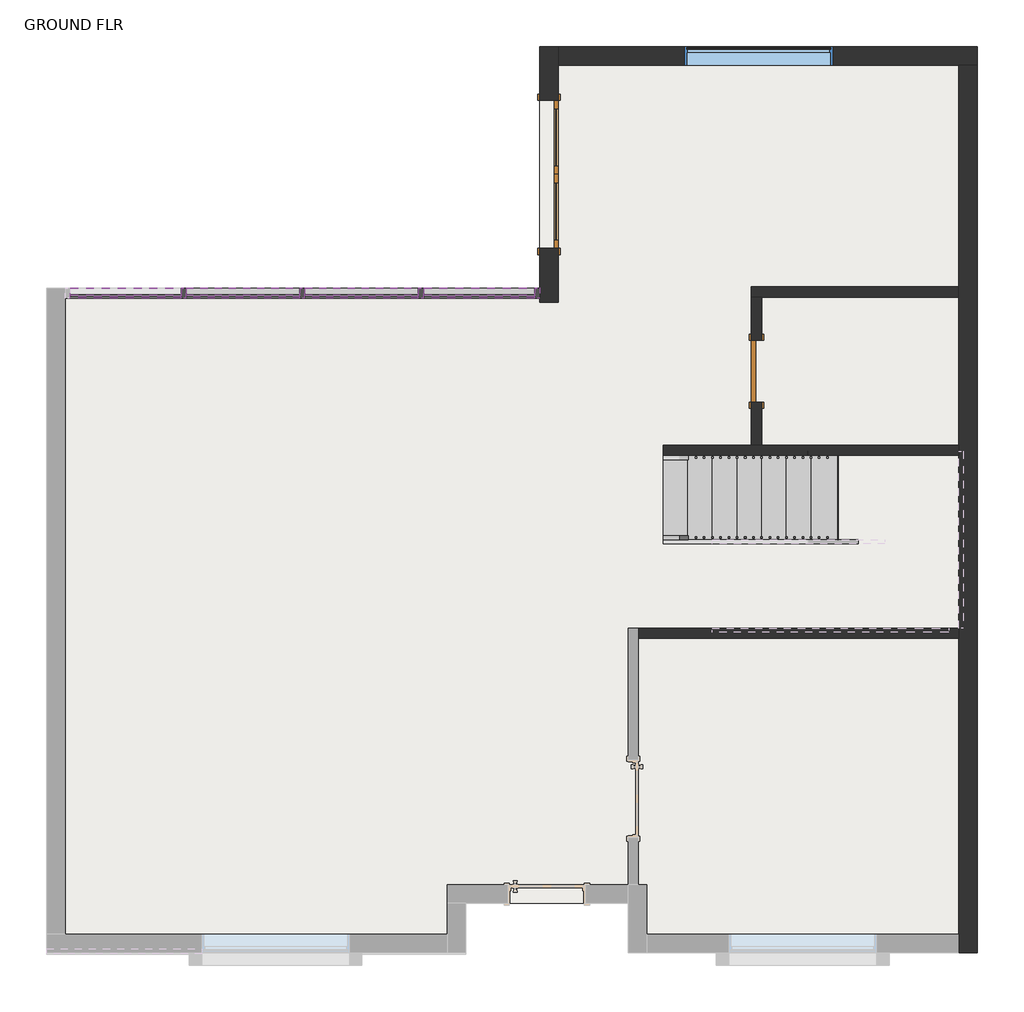
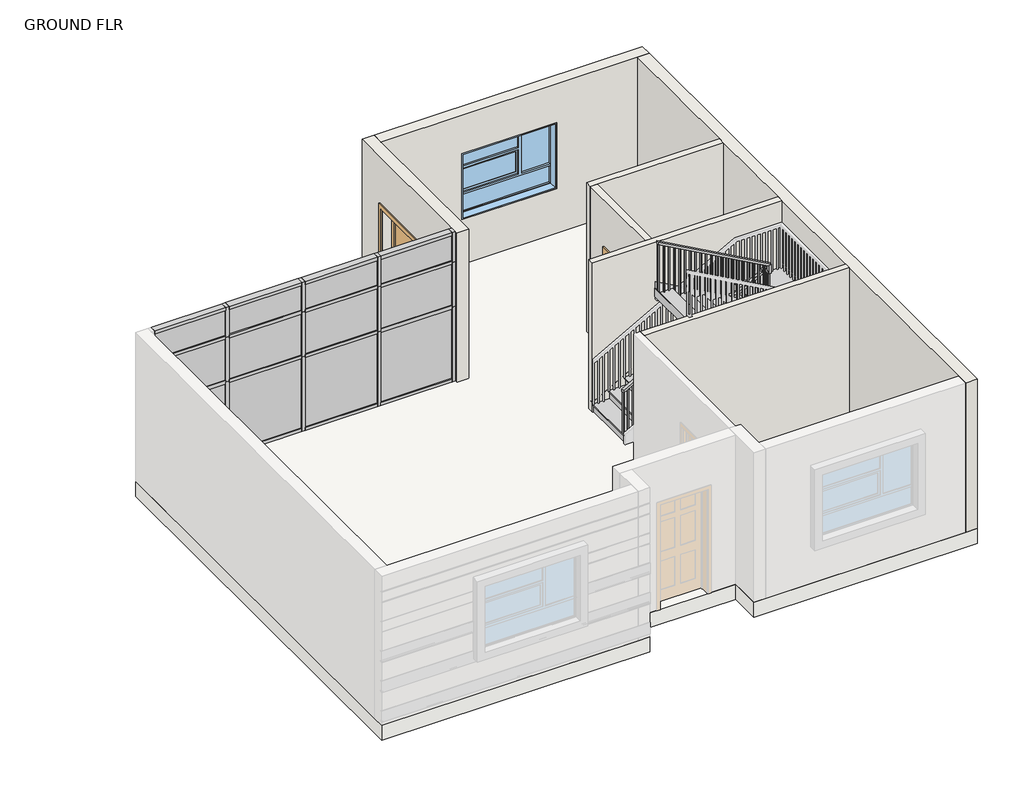
# One storey, part 3 of 4: 27 members, 12 plates, 7 walls, 2 doors, 1 railing, 1 slab, 1 stair flight, 1 window.
"""IFC4 building model written with IfcOpenShell, lengths in millimetres."""

from ifc_helpers import new_model, si_unit, frame, origin, origin_with_axes, place, context, project, spatial, polyline, outline, extrude, faceted_brep, transform, mapped, element, save
from components import door_4594e60e, door_1fe7f57d, member_bb3ab01a, member_a4baedd8, member_82905deb, member_554b6236, member_3093b26a, member_410c6227, member_6e77e263, member_4491d118, member_73c23c35, member_47bfaf8a, system_panel_glazed_499fa1d4, system_panel_glazed_0f0a4f2b, system_panel_glazed_cad8d6ff, system_panel_glazed_5760c905, system_panel_glazed_04da4e26, system_panel_glazed_82e8a1e7, stair_flight_e0aa27d8, window_511101a2

model = new_model("IFC4")

# Units and contexts
model_context = context("Model", 3, world=origin())
ifc_project = project(units=[si_unit("LENGTHUNIT", "METRE", prefix="MILLI")], contexts=[model_context])

# Site, building, storey
site = spatial("IfcSite", under=ifc_project)
building = spatial("IfcBuilding", under=site)
storey = spatial("IfcBuildingStorey", under=building, Name="GROUND FLR", Elevation=304.8)

# Doors
placement = place(None, origin())
door_shape = door_4594e60e(model_context)
element("IfcDoor", 1, ObjectType="Door-Double-Glass : 72\" x 80\"", at=placement, inside=storey, context=model_context, shape_type="MappedRepresentation", body=[
    mapped(door_shape, transform((363.8858709, 7170.3723211, 304.8), x_axis=(0.0, -1.0, 0.0), y_axis=(1.0, 0.0, 0.0), z_axis=(0.0, 0.0, 1.0))),
])
door_2_shape = door_1fe7f57d(model_context)
element("IfcDoor", 2, ObjectType="Single-Flush : bathroom flush door 2' 6\" x 7'", at=placement, inside=storey, context=model_context, shape_type="MappedRepresentation", body=[
    mapped(door_2_shape, transform((2931.6671209, 4738.3223211, 304.8), x_axis=(0.0, 1.0, 0.0), y_axis=(-1.0, 0.0, 0.0), z_axis=(0.0, 0.0, 1.0))),
])

# Members
member_shape = member_bb3ab01a(model_context)
element("IfcMember", 3, ObjectType="Rectangular Mullion : 2.5\" x 5\" rectangular", at=placement, inside=storey, context=model_context, shape_type="MappedRepresentation", body=[
    mapped(member_shape, transform((188.4671209, 5703.5223211, 3352.8), x_axis=(0.0, 0.0, 1.0), y_axis=(0.0, -1.0, 0.0), z_axis=(1.0, 0.0, 0.0))),
])
element("IfcMember", 4, ObjectType="Rectangular Mullion : 2.5\" x 5\" rectangular", at=placement, inside=storey, context=model_context, shape_type="MappedRepresentation", body=[
    mapped(member_shape, transform((-4180.332879, 5703.5223211, 3352.8), x_axis=(0.0, 0.0, 1.0), y_axis=(0.0, -1.0, 0.0), z_axis=(1.0, 0.0, 0.0))),
])
element("IfcMember", 5, ObjectType="Rectangular Mullion : 2.5\" x 5\" rectangular", at=placement, inside=storey, context=model_context, shape_type="MappedRepresentation", body=[
    mapped(member_shape, transform((-1183.1328793, 5703.5223211, 304.8), x_axis=(0.0, 0.0, -1.0), y_axis=(0.0, -1.0, 0.0), z_axis=(-1.0, 0.0, 0.0))),
])
member_2_shape = member_a4baedd8(model_context)
element("IfcMember", 6, ObjectType="Rectangular Mullion : 2.5\" x 5\" rectangular", at=placement, inside=storey, context=model_context, shape_type="MappedRepresentation", body=[
    mapped(member_2_shape, transform((-2713.4828791, 5703.5223211, 3352.8), x_axis=(0.0, 0.0, 1.0), y_axis=(0.0, -1.0, 0.0), z_axis=(1.0, 0.0, 0.0))),
])
element("IfcMember", 7, ObjectType="Rectangular Mullion : 2.5\" x 5\" rectangular", at=placement, inside=storey, context=model_context, shape_type="MappedRepresentation", body=[
    mapped(member_2_shape, transform((-1246.6328793, 5703.5223211, 3352.8), x_axis=(0.0, 0.0, 1.0), y_axis=(0.0, -1.0, 0.0), z_axis=(1.0, 0.0, 0.0))),
])
element("IfcMember", 8, ObjectType="Rectangular Mullion : 2.5\" x 5\" rectangular", at=placement, inside=storey, context=model_context, shape_type="MappedRepresentation", body=[
    mapped(member_2_shape, transform((-4116.832879, 5703.5223211, 304.8), x_axis=(0.0, 0.0, -1.0), y_axis=(0.0, -1.0, 0.0), z_axis=(-1.0, 0.0, 0.0))),
])
element("IfcMember", 9, ObjectType="Rectangular Mullion : 2.5\" x 5\" rectangular", at=placement, inside=storey, context=model_context, shape_type="MappedRepresentation", body=[
    mapped(member_2_shape, transform((-2649.9828791, 5703.5223211, 304.8), x_axis=(0.0, 0.0, -1.0), y_axis=(0.0, -1.0, 0.0), z_axis=(-1.0, 0.0, 0.0))),
])
member_3_shape = member_82905deb(model_context)
element("IfcMember", 10, ObjectType="Rectangular Mullion : 2.5\" x 5\" rectangular", at=placement, inside=storey, context=model_context, shape_type="MappedRepresentation", body=[
    mapped(member_3_shape, transform((-4148.582879, 5703.5223211, 304.8), x_axis=(1.0, 0.0, 0.0), y_axis=(0.0, -1.0, 0.0), z_axis=(0.0, 0.0, -1.0))),
])
element("IfcMember", 11, ObjectType="Rectangular Mullion : 2.5\" x 5\" rectangular", at=placement, inside=storey, context=model_context, shape_type="MappedRepresentation", body=[
    mapped(member_3_shape, transform((-2681.7328791, 5703.5223211, 304.8), x_axis=(1.0, 0.0, 0.0), y_axis=(0.0, -1.0, 0.0), z_axis=(0.0, 0.0, -1.0))),
])
element("IfcMember", 12, ObjectType="Rectangular Mullion : 2.5\" x 5\" rectangular", at=placement, inside=storey, context=model_context, shape_type="MappedRepresentation", body=[
    mapped(member_3_shape, transform((-1214.8828793, 5703.5223211, 304.8), x_axis=(1.0, 0.0, 0.0), y_axis=(0.0, -1.0, 0.0), z_axis=(0.0, 0.0, -1.0))),
])
member_4_shape = member_554b6236(model_context)
element("IfcMember", 13, ObjectType="Rectangular Mullion : 2.5\" x 5\" rectangular", at=placement, inside=storey, context=model_context, shape_type="MappedRepresentation", body=[
    mapped(member_4_shape, transform((-4180.332879, 5703.5223211, 1828.8), x_axis=(0.0, 0.0, 1.0), y_axis=(0.0, -1.0, 0.0), z_axis=(1.0, 0.0, 0.0))),
])
element("IfcMember", 14, ObjectType="Rectangular Mullion : 2.5\" x 5\" rectangular", at=placement, inside=storey, context=model_context, shape_type="MappedRepresentation", body=[
    mapped(member_4_shape, transform((188.4671209, 5703.5223211, 1828.8), x_axis=(0.0, 0.0, 1.0), y_axis=(0.0, -1.0, 0.0), z_axis=(1.0, 0.0, 0.0))),
])
element("IfcMember", 15, ObjectType="Rectangular Mullion : 2.5\" x 5\" rectangular", at=placement, inside=storey, context=model_context, shape_type="MappedRepresentation", body=[
    mapped(member_4_shape, transform((-4180.332879, 5703.5223211, 2743.2), x_axis=(0.0, 0.0, 1.0), y_axis=(0.0, -1.0, 0.0), z_axis=(1.0, 0.0, 0.0))),
])
element("IfcMember", 16, ObjectType="Rectangular Mullion : 2.5\" x 5\" rectangular", at=placement, inside=storey, context=model_context, shape_type="MappedRepresentation", body=[
    mapped(member_4_shape, transform((188.4671209, 5703.5223211, 2743.2), x_axis=(0.0, 0.0, 1.0), y_axis=(0.0, -1.0, 0.0), z_axis=(1.0, 0.0, 0.0))),
])
member_5_shape = member_3093b26a(model_context)
element("IfcMember", 17, ObjectType="Rectangular Mullion : 2.5\" x 5\" rectangular", at=placement, inside=storey, context=model_context, shape_type="MappedRepresentation", body=[
    mapped(member_5_shape, transform((-2713.4828791, 5703.5223211, 1828.8), x_axis=(0.0, 0.0, 1.0), y_axis=(0.0, -1.0, 0.0), z_axis=(1.0, 0.0, 0.0))),
])
element("IfcMember", 18, ObjectType="Rectangular Mullion : 2.5\" x 5\" rectangular", at=placement, inside=storey, context=model_context, shape_type="MappedRepresentation", body=[
    mapped(member_5_shape, transform((-1246.6328793, 5703.5223211, 1828.8), x_axis=(0.0, 0.0, 1.0), y_axis=(0.0, -1.0, 0.0), z_axis=(1.0, 0.0, 0.0))),
])
element("IfcMember", 19, ObjectType="Rectangular Mullion : 2.5\" x 5\" rectangular", at=placement, inside=storey, context=model_context, shape_type="MappedRepresentation", body=[
    mapped(member_5_shape, transform((-2713.4828791, 5703.5223211, 2743.2), x_axis=(0.0, 0.0, 1.0), y_axis=(0.0, -1.0, 0.0), z_axis=(1.0, 0.0, 0.0))),
])
element("IfcMember", 20, ObjectType="Rectangular Mullion : 2.5\" x 5\" rectangular", at=placement, inside=storey, context=model_context, shape_type="MappedRepresentation", body=[
    mapped(member_5_shape, transform((-1246.6328793, 5703.5223211, 2743.2), x_axis=(0.0, 0.0, 1.0), y_axis=(0.0, -1.0, 0.0), z_axis=(1.0, 0.0, 0.0))),
])
member_6_shape = member_410c6227(model_context)
element("IfcMember", 21, ObjectType="Rectangular Mullion : 2.5\" x 5\" rectangular", at=placement, inside=storey, context=model_context, shape_type="MappedRepresentation", body=[
    mapped(member_6_shape, transform((-4148.582879, 5703.5223211, 1828.8), x_axis=(1.0, 0.0, 0.0), y_axis=(0.0, -1.0, 0.0), z_axis=(0.0, 0.0, -1.0))),
])
element("IfcMember", 22, ObjectType="Rectangular Mullion : 2.5\" x 5\" rectangular", at=placement, inside=storey, context=model_context, shape_type="MappedRepresentation", body=[
    mapped(member_6_shape, transform((-2681.7328791, 5703.5223211, 1828.8), x_axis=(1.0, 0.0, 0.0), y_axis=(0.0, -1.0, 0.0), z_axis=(0.0, 0.0, -1.0))),
])
element("IfcMember", 23, ObjectType="Rectangular Mullion : 2.5\" x 5\" rectangular", at=placement, inside=storey, context=model_context, shape_type="MappedRepresentation", body=[
    mapped(member_6_shape, transform((-1214.8828793, 5703.5223211, 1828.8), x_axis=(1.0, 0.0, 0.0), y_axis=(0.0, -1.0, 0.0), z_axis=(0.0, 0.0, -1.0))),
])
member_7_shape = member_6e77e263(model_context)
element("IfcMember", 24, ObjectType="Rectangular Mullion : 2.5\" x 5\" rectangular", at=placement, inside=storey, context=model_context, shape_type="MappedRepresentation", body=[
    mapped(member_7_shape, transform((-4148.582879, 5703.5223211, 2743.2), x_axis=(1.0, 0.0, 0.0), y_axis=(0.0, -1.0, 0.0), z_axis=(0.0, 0.0, -1.0))),
])
element("IfcMember", 25, ObjectType="Rectangular Mullion : 2.5\" x 5\" rectangular", at=placement, inside=storey, context=model_context, shape_type="MappedRepresentation", body=[
    mapped(member_7_shape, transform((-2681.7328791, 5703.5223211, 2743.2), x_axis=(1.0, 0.0, 0.0), y_axis=(0.0, -1.0, 0.0), z_axis=(0.0, 0.0, -1.0))),
])
element("IfcMember", 26, ObjectType="Rectangular Mullion : 2.5\" x 5\" rectangular", at=placement, inside=storey, context=model_context, shape_type="MappedRepresentation", body=[
    mapped(member_7_shape, transform((-1214.8828793, 5703.5223211, 2743.2), x_axis=(1.0, 0.0, 0.0), y_axis=(0.0, -1.0, 0.0), z_axis=(0.0, 0.0, -1.0))),
])
member_8_shape = member_4491d118(model_context)
element("IfcMember", 27, ObjectType="Rectangular Mullion : 2.5\" x 5\" rectangular", at=placement, inside=storey, context=model_context, shape_type="MappedRepresentation", body=[
    mapped(member_8_shape, transform((251.9671209, 5703.5223211, 304.8), x_axis=(1.0, 0.0, 0.0), y_axis=(0.0, -1.0, 0.0), z_axis=(0.0, 0.0, -1.0))),
])
member_9_shape = member_73c23c35(model_context)
element("IfcMember", 28, ObjectType="Rectangular Mullion : 2.5\" x 5\" rectangular", at=placement, inside=storey, context=model_context, shape_type="MappedRepresentation", body=[
    mapped(member_9_shape, transform((251.9671209, 5703.5223211, 1828.8), x_axis=(1.0, 0.0, 0.0), y_axis=(0.0, -1.0, 0.0), z_axis=(0.0, 0.0, -1.0))),
])
member_10_shape = member_47bfaf8a(model_context)
element("IfcMember", 29, ObjectType="Rectangular Mullion : 2.5\" x 5\" rectangular", at=placement, inside=storey, context=model_context, shape_type="MappedRepresentation", body=[
    mapped(member_10_shape, transform((251.9671209, 5703.5223211, 2743.2), x_axis=(1.0, 0.0, 0.0), y_axis=(0.0, -1.0, 0.0), z_axis=(0.0, 0.0, -1.0))),
])

# Plates
system_panel_glazed_shape = system_panel_glazed_499fa1d4(model_context)
element("IfcPlate", 30, ObjectType="System Panel : Glazed", at=placement, inside=storey, context=model_context, shape_type="MappedRepresentation", body=[
    mapped(system_panel_glazed_shape, transform((-4866.1328791, 5703.5223211, 368.3), x_axis=(1.0, 0.0, 0.0), y_axis=(0.0, 1.0, 0.0), z_axis=(0.0, 0.0, 1.0))),
])
element("IfcPlate", 31, ObjectType="System Panel : Glazed", at=placement, inside=storey, context=model_context, shape_type="MappedRepresentation", body=[
    mapped(system_panel_glazed_shape, transform((-497.3328792, 5703.5223211, 368.3), x_axis=(1.0, 0.0, 0.0), y_axis=(0.0, 1.0, 0.0), z_axis=(0.0, 0.0, 1.0))),
])
system_panel_glazed_2_shape = system_panel_glazed_0f0a4f2b(model_context)
element("IfcPlate", 32, ObjectType="System Panel : Glazed", at=placement, inside=storey, context=model_context, shape_type="MappedRepresentation", body=[
    mapped(system_panel_glazed_2_shape, transform((-3415.1578791, 5703.5223211, 368.3), x_axis=(1.0, 0.0, 0.0), y_axis=(0.0, 1.0, 0.0), z_axis=(0.0, 0.0, 1.0))),
])
element("IfcPlate", 33, ObjectType="System Panel : Glazed", at=placement, inside=storey, context=model_context, shape_type="MappedRepresentation", body=[
    mapped(system_panel_glazed_2_shape, transform((-1948.3078792, 5703.5223211, 368.3), x_axis=(1.0, 0.0, 0.0), y_axis=(0.0, 1.0, 0.0), z_axis=(0.0, 0.0, 1.0))),
])
system_panel_glazed_3_shape = system_panel_glazed_cad8d6ff(model_context)
element("IfcPlate", 34, ObjectType="System Panel : Glazed", at=placement, inside=storey, context=model_context, shape_type="MappedRepresentation", body=[
    mapped(system_panel_glazed_3_shape, transform((-4866.1328791, 5703.5223211, 1860.55), x_axis=(1.0, 0.0, 0.0), y_axis=(0.0, 1.0, 0.0), z_axis=(0.0, 0.0, 1.0))),
])
element("IfcPlate", 35, ObjectType="System Panel : Glazed", at=placement, inside=storey, context=model_context, shape_type="MappedRepresentation", body=[
    mapped(system_panel_glazed_3_shape, transform((-497.3328792, 5703.5223211, 1860.55), x_axis=(1.0, 0.0, 0.0), y_axis=(0.0, 1.0, 0.0), z_axis=(0.0, 0.0, 1.0))),
])
system_panel_glazed_4_shape = system_panel_glazed_5760c905(model_context)
element("IfcPlate", 36, ObjectType="System Panel : Glazed", at=placement, inside=storey, context=model_context, shape_type="MappedRepresentation", body=[
    mapped(system_panel_glazed_4_shape, transform((-3415.1578791, 5703.5223211, 1860.55), x_axis=(1.0, 0.0, 0.0), y_axis=(0.0, 1.0, 0.0), z_axis=(0.0, 0.0, 1.0))),
])
element("IfcPlate", 37, ObjectType="System Panel : Glazed", at=placement, inside=storey, context=model_context, shape_type="MappedRepresentation", body=[
    mapped(system_panel_glazed_4_shape, transform((-1948.3078792, 5703.5223211, 1860.55), x_axis=(1.0, 0.0, 0.0), y_axis=(0.0, 1.0, 0.0), z_axis=(0.0, 0.0, 1.0))),
])
system_panel_glazed_5_shape = system_panel_glazed_04da4e26(model_context)
element("IfcPlate", 38, ObjectType="System Panel : Glazed", at=placement, inside=storey, context=model_context, shape_type="MappedRepresentation", body=[
    mapped(system_panel_glazed_5_shape, transform((-4866.1328791, 5703.5223211, 2774.95), x_axis=(1.0, 0.0, 0.0), y_axis=(0.0, 1.0, 0.0), z_axis=(0.0, 0.0, 1.0))),
])
element("IfcPlate", 39, ObjectType="System Panel : Glazed", at=placement, inside=storey, context=model_context, shape_type="MappedRepresentation", body=[
    mapped(system_panel_glazed_5_shape, transform((-497.3328792, 5703.5223211, 2774.95), x_axis=(1.0, 0.0, 0.0), y_axis=(0.0, 1.0, 0.0), z_axis=(0.0, 0.0, 1.0))),
])
system_panel_glazed_6_shape = system_panel_glazed_82e8a1e7(model_context)
element("IfcPlate", 40, ObjectType="System Panel : Glazed", at=placement, inside=storey, context=model_context, shape_type="MappedRepresentation", body=[
    mapped(system_panel_glazed_6_shape, transform((-3415.1578791, 5703.5223211, 2774.95), x_axis=(1.0, 0.0, 0.0), y_axis=(0.0, 1.0, 0.0), z_axis=(0.0, 0.0, 1.0))),
])
element("IfcPlate", 41, ObjectType="System Panel : Glazed", at=placement, inside=storey, context=model_context, shape_type="MappedRepresentation", body=[
    mapped(system_panel_glazed_6_shape, transform((-1948.3078792, 5703.5223211, 2774.95), x_axis=(1.0, 0.0, 0.0), y_axis=(0.0, 1.0, 0.0), z_axis=(0.0, 0.0, 1.0))),
])

# Railing
element("IfcRailing", 42, ObjectType="Handrail - Rectangular", at=placement, inside=storey, context=model_context, shape_type="SolidModel", body=[
    faceted_brep([(1775.9671209, 2706.3223211, 1388.5333333), (1775.9671209, 2706.3223211, 1330.420221), (1775.9671209, 2655.5223211, 1330.420221), (1775.9671209, 2655.5223211, 1388.5333333), (4442.9671209, 2706.3223211, 2870.2), (4493.7671209, 2706.3223211, 2840.3091099), (4493.7671209, 2655.5223211, 2840.3091099), (4442.9671209, 2655.5223211, 2870.2), (4442.9671209, 2706.3223211, 2912.5333333), (4493.7671209, 2706.3223211, 2861.7333333), (4493.7671209, 2655.5223211, 2861.7333333), (4442.9671209, 2655.5223211, 2912.5333333), (4569.9671209, 2706.3223211, 2912.5333333), (4569.9671209, 2706.3223211, 2861.7333333), (4519.1671209, 2655.5223211, 2861.7333333), (4519.1671209, 2655.5223211, 2912.5333333), (4569.9671209, 2604.7223211, 2912.5333333), (4519.1671209, 2604.7223211, 2912.5333333), (4519.1671209, 2553.9223211, 2861.7333333), (4569.9671209, 2553.9223211, 2861.7333333)], [[[0, 1, 2, 3]], [[1, 0, 4, 5]], [[2, 1, 5, 6]], [[3, 2, 6, 7]], [[0, 3, 7, 4]], [[5, 4, 8, 9]], [[6, 5, 9, 10]], [[7, 6, 10, 11]], [[4, 7, 11, 8]], [[9, 8, 12, 13]], [[10, 9, 13, 14]], [[11, 10, 14, 15]], [[8, 11, 15, 12]], [[16, 17, 18, 19]], [[13, 12, 16, 19]], [[14, 13, 19, 18]], [[15, 14, 18, 17]], [[12, 15, 17, 16]]]),
    faceted_brep([(4569.9671209, 2604.7223211, 2912.5333333), (4569.9671209, 2553.9223211, 2861.7333333), (4519.1671209, 2553.9223211, 2861.7333333), (4519.1671209, 2604.7223211, 2912.5333333), (4569.9671209, 2604.7223211, 3053.6444444), (4519.1671209, 2604.7223211, 3023.7535543), (4519.1671209, 2553.9223211, 3023.7535543), (4569.9671209, 2553.9223211, 3053.6444444)], [[[0, 1, 2, 3]], [[4, 5, 6, 7]], [[1, 0, 4, 7]], [[2, 1, 7, 6]], [[3, 2, 6, 5]], [[0, 3, 5, 4]]]),
    faceted_brep([(4569.9671209, 2553.9223211, 3053.6444444), (4519.1671209, 2553.9223211, 3023.7535543), (4519.1671209, 2604.7223211, 3023.7535543), (4569.9671209, 2604.7223211, 3053.6444444), (2385.5671209, 2553.9223211, 4267.2), (2385.5671209, 2604.7223211, 4267.2), (2385.5671209, 2604.7223211, 4209.0868876), (2385.5671209, 2553.9223211, 4209.0868876)], [[[0, 1, 2, 3]], [[4, 5, 6, 7]], [[1, 0, 4, 7]], [[2, 1, 7, 6]], [[3, 2, 6, 5]], [[0, 3, 5, 4]]]),
    extrude(outline(polyline([(4189.6841099, 2420.4921209), (4200.2674432, 2401.4421209), (3183.4666667, 2401.4421209), (3183.4666667, 2420.4921209), (4189.6841099, 2420.4921209)])), frame((0.0, 2569.7973211, 0.0), z_axis=(0.0, 1.0, 0.0), x_axis=(0.0, 0.0, 1.0)), (0.0, 0.0, 1.0), 19.05),
    extrude(outline(polyline([(4133.2396654, 2522.0921209), (4143.8229988, 2503.0421209), (3183.4666667, 2503.0421209), (3183.4666667, 2522.0921209), (4133.2396654, 2522.0921209)])), frame((0.0, 2569.7973211, 0.0), z_axis=(0.0, 1.0, 0.0), x_axis=(0.0, 0.0, 1.0)), (0.0, 0.0, 1.0), 19.05),
    extrude(outline(polyline([(4076.795221, 2623.6921209), (4087.3785543, 2604.6421209), (3183.4666667, 2604.6421209), (3183.4666667, 2623.6921209), (4076.795221, 2623.6921209)])), frame((0.0, 2569.7973211, 0.0), z_axis=(0.0, 1.0, 0.0), x_axis=(0.0, 0.0, 1.0)), (0.0, 0.0, 1.0), 19.05),
    extrude(outline(polyline([(4020.3507765, 2725.2921209), (4030.9341099, 2706.2421209), (3014.1333333, 2706.2421209), (3014.1333333, 2725.2921209), (4020.3507765, 2725.2921209)])), frame((0.0, 2569.7973211, 0.0), z_axis=(0.0, 1.0, 0.0), x_axis=(0.0, 0.0, 1.0)), (0.0, 0.0, 1.0), 19.05),
    extrude(outline(polyline([(3963.9063321, 2826.8921209), (3974.4896654, 2807.8421209), (3014.1333333, 2807.8421209), (3014.1333333, 2826.8921209), (3963.9063321, 2826.8921209)])), frame((0.0, 2569.7973211, 0.0), z_axis=(0.0, 1.0, 0.0), x_axis=(0.0, 0.0, 1.0)), (0.0, 0.0, 1.0), 19.05),
    extrude(outline(polyline([(3907.4618876, 2928.4921209), (3918.045221, 2909.4421209), (3014.1333333, 2909.4421209), (3014.1333333, 2928.4921209), (3907.4618876, 2928.4921209)])), frame((0.0, 2569.7973211, 0.0), z_axis=(0.0, 1.0, 0.0), x_axis=(0.0, 0.0, 1.0)), (0.0, 0.0, 1.0), 19.05),
    extrude(outline(polyline([(3851.0174432, 3030.0921209), (3861.6007765, 3011.0421209), (2844.8, 3011.0421209), (2844.8, 3030.0921209), (3851.0174432, 3030.0921209)])), frame((0.0, 2569.7973211, 0.0), z_axis=(0.0, 1.0, 0.0), x_axis=(0.0, 0.0, 1.0)), (0.0, 0.0, 1.0), 19.05),
    extrude(outline(polyline([(3794.5729988, 3131.6921209), (3805.1563321, 3112.6421209), (2844.8, 3112.6421209), (2844.8, 3131.6921209), (3794.5729988, 3131.6921209)])), frame((0.0, 2569.7973211, 0.0), z_axis=(0.0, 1.0, 0.0), x_axis=(0.0, 0.0, 1.0)), (0.0, 0.0, 1.0), 19.05),
    extrude(outline(polyline([(3738.1285543, 3233.2921209), (3748.7118876, 3214.2421209), (2844.8, 3214.2421209), (2844.8, 3233.2921209), (3738.1285543, 3233.2921209)])), frame((0.0, 2569.7973211, 0.0), z_axis=(0.0, 1.0, 0.0), x_axis=(0.0, 0.0, 1.0)), (0.0, 0.0, 1.0), 19.05),
    extrude(outline(polyline([(3681.6841099, 3334.8921209), (3692.2674432, 3315.8421209), (2675.4666667, 3315.8421209), (2675.4666667, 3334.8921209), (3681.6841099, 3334.8921209)])), frame((0.0, 2569.7973211, 0.0), z_axis=(0.0, 1.0, 0.0), x_axis=(0.0, 0.0, 1.0)), (0.0, 0.0, 1.0), 19.05),
    extrude(outline(polyline([(3625.2396654, 3436.4921209), (3635.8229988, 3417.4421209), (2675.4666667, 3417.4421209), (2675.4666667, 3436.4921209), (3625.2396654, 3436.4921209)])), frame((0.0, 2569.7973211, 0.0), z_axis=(0.0, 1.0, 0.0), x_axis=(0.0, 0.0, 1.0)), (0.0, 0.0, 1.0), 19.05),
    extrude(outline(polyline([(3568.795221, 3538.0921209), (3579.3785543, 3519.0421209), (2675.4666667, 3519.0421209), (2675.4666667, 3538.0921209), (3568.795221, 3538.0921209)])), frame((0.0, 2569.7973211, 0.0), z_axis=(0.0, 1.0, 0.0), x_axis=(0.0, 0.0, 1.0)), (0.0, 0.0, 1.0), 19.05),
    extrude(outline(polyline([(3512.3507765, 3639.6921209), (3522.9341099, 3620.6421209), (2506.1333333, 3620.6421209), (2506.1333333, 3639.6921209), (3512.3507765, 3639.6921209)])), frame((0.0, 2569.7973211, 0.0), z_axis=(0.0, 1.0, 0.0), x_axis=(0.0, 0.0, 1.0)), (0.0, 0.0, 1.0), 19.05),
    extrude(outline(polyline([(3455.9063321, 3741.2921209), (3466.4896654, 3722.2421209), (2506.1333333, 3722.2421209), (2506.1333333, 3741.2921209), (3455.9063321, 3741.2921209)])), frame((0.0, 2569.7973211, 0.0), z_axis=(0.0, 1.0, 0.0), x_axis=(0.0, 0.0, 1.0)), (0.0, 0.0, 1.0), 19.05),
    extrude(outline(polyline([(3399.4618876, 3842.8921209), (3410.045221, 3823.8421209), (2506.1333333, 3823.8421209), (2506.1333333, 3842.8921209), (3399.4618876, 3842.8921209)])), frame((0.0, 2569.7973211, 0.0), z_axis=(0.0, 1.0, 0.0), x_axis=(0.0, 0.0, 1.0)), (0.0, 0.0, 1.0), 19.05),
    extrude(outline(polyline([(3343.0174432, 3944.4921209), (3353.6007765, 3925.4421209), (2336.8, 3925.4421209), (2336.8, 3944.4921209), (3343.0174432, 3944.4921209)])), frame((0.0, 2569.7973211, 0.0), z_axis=(0.0, 1.0, 0.0), x_axis=(0.0, 0.0, 1.0)), (0.0, 0.0, 1.0), 19.05),
    extrude(outline(polyline([(3286.5729988, 4046.0921209), (3297.1563321, 4027.0421209), (2336.8, 4027.0421209), (2336.8, 4046.0921209), (3286.5729988, 4046.0921209)])), frame((0.0, 2569.7973211, 0.0), z_axis=(0.0, 1.0, 0.0), x_axis=(0.0, 0.0, 1.0)), (0.0, 0.0, 1.0), 19.05),
    extrude(outline(polyline([(3230.1285543, 4147.6921209), (3240.7118876, 4128.6421209), (2336.8, 4128.6421209), (2336.8, 4147.6921209), (3230.1285543, 4147.6921209)])), frame((0.0, 2569.7973211, 0.0), z_axis=(0.0, 1.0, 0.0), x_axis=(0.0, 0.0, 1.0)), (0.0, 0.0, 1.0), 19.05),
    extrude(outline(polyline([(3173.6841099, 4249.2921209), (3184.2674432, 4230.2421209), (2167.4666667, 4230.2421209), (2167.4666667, 4249.2921209), (3173.6841099, 4249.2921209)])), frame((0.0, 2569.7973211, 0.0), z_axis=(0.0, 1.0, 0.0), x_axis=(0.0, 0.0, 1.0)), (0.0, 0.0, 1.0), 19.05),
    extrude(outline(polyline([(3117.2396654, 4350.8921209), (3127.8229988, 4331.8421209), (2167.4666667, 4331.8421209), (2167.4666667, 4350.8921209), (3117.2396654, 4350.8921209)])), frame((0.0, 2569.7973211, 0.0), z_axis=(0.0, 1.0, 0.0), x_axis=(0.0, 0.0, 1.0)), (0.0, 0.0, 1.0), 19.05),
    extrude(outline(polyline([(3060.795221, 4452.4921209), (3071.3785543, 4433.4421209), (2167.4666667, 4433.4421209), (2167.4666667, 4452.4921209), (3060.795221, 4452.4921209)])), frame((0.0, 2569.7973211, 0.0), z_axis=(0.0, 1.0, 0.0), x_axis=(0.0, 0.0, 1.0)), (0.0, 0.0, 1.0), 19.05),
    extrude(outline(polyline([(4509.6421209, 2671.3973211), (4509.6421209, 2690.4473211), (4528.6921209, 2690.4473211), (4528.6921209, 2671.3973211), (4509.6421209, 2671.3973211)])), frame((0.0, 0.0, 1998.1333333), z_axis=(0.0, 0.0, 1.0), x_axis=(1.0, 0.0, 0.0)), (0.0, 0.0, 1.0), 863.6),
    extrude(outline(polyline([(2803.2674432, 4427.0921209), (2792.6841099, 4408.0421209), (1828.8, 4408.0421209), (1828.8, 4427.0921209), (2803.2674432, 4427.0921209)])), frame((0.0, 2671.3973211, 0.0), z_axis=(0.0, 1.0, 0.0), x_axis=(0.0, 0.0, 1.0)), (0.0, 0.0, 1.0), 19.05),
    extrude(outline(polyline([(2746.8229988, 4325.4921209), (2736.2396654, 4306.4421209), (1828.8, 4306.4421209), (1828.8, 4325.4921209), (2746.8229988, 4325.4921209)])), frame((0.0, 2671.3973211, 0.0), z_axis=(0.0, 1.0, 0.0), x_axis=(0.0, 0.0, 1.0)), (0.0, 0.0, 1.0), 19.05),
    extrude(outline(polyline([(2690.3785543, 4223.8921209), (2679.795221, 4204.8421209), (1828.8, 4204.8421209), (1828.8, 4223.8921209), (2690.3785543, 4223.8921209)])), frame((0.0, 2671.3973211, 0.0), z_axis=(0.0, 1.0, 0.0), x_axis=(0.0, 0.0, 1.0)), (0.0, 0.0, 1.0), 19.05),
    extrude(outline(polyline([(2633.9341099, 4122.2921209), (2623.3507765, 4103.2421209), (1659.4666667, 4103.2421209), (1659.4666667, 4122.2921209), (2633.9341099, 4122.2921209)])), frame((0.0, 2671.3973211, 0.0), z_axis=(0.0, 1.0, 0.0), x_axis=(0.0, 0.0, 1.0)), (0.0, 0.0, 1.0), 19.05),
    extrude(outline(polyline([(2577.4896654, 4020.6921209), (2566.9063321, 4001.6421209), (1659.4666667, 4001.6421209), (1659.4666667, 4020.6921209), (2577.4896654, 4020.6921209)])), frame((0.0, 2671.3973211, 0.0), z_axis=(0.0, 1.0, 0.0), x_axis=(0.0, 0.0, 1.0)), (0.0, 0.0, 1.0), 19.05),
    extrude(outline(polyline([(2521.045221, 3919.0921209), (2510.4618876, 3900.0421209), (1659.4666667, 3900.0421209), (1659.4666667, 3919.0921209), (2521.045221, 3919.0921209)])), frame((0.0, 2671.3973211, 0.0), z_axis=(0.0, 1.0, 0.0), x_axis=(0.0, 0.0, 1.0)), (0.0, 0.0, 1.0), 19.05),
    extrude(outline(polyline([(2464.6007765, 3817.4921209), (2454.0174432, 3798.4421209), (1490.1333333, 3798.4421209), (1490.1333333, 3817.4921209), (2464.6007765, 3817.4921209)])), frame((0.0, 2671.3973211, 0.0), z_axis=(0.0, 1.0, 0.0), x_axis=(0.0, 0.0, 1.0)), (0.0, 0.0, 1.0), 19.05),
    extrude(outline(polyline([(2408.1563321, 3715.8921209), (2397.5729988, 3696.8421209), (1490.1333333, 3696.8421209), (1490.1333333, 3715.8921209), (2408.1563321, 3715.8921209)])), frame((0.0, 2671.3973211, 0.0), z_axis=(0.0, 1.0, 0.0), x_axis=(0.0, 0.0, 1.0)), (0.0, 0.0, 1.0), 19.05),
    extrude(outline(polyline([(2351.7118876, 3614.2921209), (2341.1285543, 3595.2421209), (1490.1333333, 3595.2421209), (1490.1333333, 3614.2921209), (2351.7118876, 3614.2921209)])), frame((0.0, 2671.3973211, 0.0), z_axis=(0.0, 1.0, 0.0), x_axis=(0.0, 0.0, 1.0)), (0.0, 0.0, 1.0), 19.05),
    extrude(outline(polyline([(2295.2674432, 3512.6921209), (2284.6841099, 3493.6421209), (1320.8, 3493.6421209), (1320.8, 3512.6921209), (2295.2674432, 3512.6921209)])), frame((0.0, 2671.3973211, 0.0), z_axis=(0.0, 1.0, 0.0), x_axis=(0.0, 0.0, 1.0)), (0.0, 0.0, 1.0), 19.05),
    extrude(outline(polyline([(2238.8229988, 3411.0921209), (2228.2396654, 3392.0421209), (1320.8, 3392.0421209), (1320.8, 3411.0921209), (2238.8229988, 3411.0921209)])), frame((0.0, 2671.3973211, 0.0), z_axis=(0.0, 1.0, 0.0), x_axis=(0.0, 0.0, 1.0)), (0.0, 0.0, 1.0), 19.05),
    extrude(outline(polyline([(2182.3785543, 3309.4921209), (2171.795221, 3290.4421209), (1320.8, 3290.4421209), (1320.8, 3309.4921209), (2182.3785543, 3309.4921209)])), frame((0.0, 2671.3973211, 0.0), z_axis=(0.0, 1.0, 0.0), x_axis=(0.0, 0.0, 1.0)), (0.0, 0.0, 1.0), 19.05),
    extrude(outline(polyline([(2125.9341099, 3207.8921209), (2115.3507765, 3188.8421209), (1151.4666667, 3188.8421209), (1151.4666667, 3207.8921209), (2125.9341099, 3207.8921209)])), frame((0.0, 2671.3973211, 0.0), z_axis=(0.0, 1.0, 0.0), x_axis=(0.0, 0.0, 1.0)), (0.0, 0.0, 1.0), 19.05),
    extrude(outline(polyline([(2069.4896654, 3106.2921209), (2058.9063321, 3087.2421209), (1151.4666667, 3087.2421209), (1151.4666667, 3106.2921209), (2069.4896654, 3106.2921209)])), frame((0.0, 2671.3973211, 0.0), z_axis=(0.0, 1.0, 0.0), x_axis=(0.0, 0.0, 1.0)), (0.0, 0.0, 1.0), 19.05),
    extrude(outline(polyline([(2013.045221, 3004.6921209), (2002.4618876, 2985.6421209), (1151.4666667, 2985.6421209), (1151.4666667, 3004.6921209), (2013.045221, 3004.6921209)])), frame((0.0, 2671.3973211, 0.0), z_axis=(0.0, 1.0, 0.0), x_axis=(0.0, 0.0, 1.0)), (0.0, 0.0, 1.0), 19.05),
    extrude(outline(polyline([(1956.6007765, 2903.0921209), (1946.0174432, 2884.0421209), (982.1333333, 2884.0421209), (982.1333333, 2903.0921209), (1956.6007765, 2903.0921209)])), frame((0.0, 2671.3973211, 0.0), z_axis=(0.0, 1.0, 0.0), x_axis=(0.0, 0.0, 1.0)), (0.0, 0.0, 1.0), 19.05),
    extrude(outline(polyline([(1900.1563321, 2801.4921209), (1889.5729988, 2782.4421209), (982.1333333, 2782.4421209), (982.1333333, 2801.4921209), (1900.1563321, 2801.4921209)])), frame((0.0, 2671.3973211, 0.0), z_axis=(0.0, 1.0, 0.0), x_axis=(0.0, 0.0, 1.0)), (0.0, 0.0, 1.0), 19.05),
    extrude(outline(polyline([(1843.7118876, 2699.8921209), (1833.1285543, 2680.8421209), (982.1333333, 2680.8421209), (982.1333333, 2699.8921209), (1843.7118876, 2699.8921209)])), frame((0.0, 2671.3973211, 0.0), z_axis=(0.0, 1.0, 0.0), x_axis=(0.0, 0.0, 1.0)), (0.0, 0.0, 1.0), 19.05),
    extrude(outline(polyline([(1787.2674432, 2598.2921209), (1776.6841099, 2579.2421209), (812.8, 2579.2421209), (812.8, 2598.2921209), (1787.2674432, 2598.2921209)])), frame((0.0, 2671.3973211, 0.0), z_axis=(0.0, 1.0, 0.0), x_axis=(0.0, 0.0, 1.0)), (0.0, 0.0, 1.0), 19.05),
    extrude(outline(polyline([(1730.8229988, 2496.6921209), (1720.2396654, 2477.6421209), (812.8, 2477.6421209), (812.8, 2496.6921209), (1730.8229988, 2496.6921209)])), frame((0.0, 2671.3973211, 0.0), z_axis=(0.0, 1.0, 0.0), x_axis=(0.0, 0.0, 1.0)), (0.0, 0.0, 1.0), 19.05),
    extrude(outline(polyline([(1674.3785543, 2395.0921209), (1663.795221, 2376.0421209), (812.8, 2376.0421209), (812.8, 2395.0921209), (1674.3785543, 2395.0921209)])), frame((0.0, 2671.3973211, 0.0), z_axis=(0.0, 1.0, 0.0), x_axis=(0.0, 0.0, 1.0)), (0.0, 0.0, 1.0), 19.05),
    extrude(outline(polyline([(1617.9341099, 2293.4921209), (1607.3507765, 2274.4421209), (643.4666667, 2274.4421209), (643.4666667, 2293.4921209), (1617.9341099, 2293.4921209)])), frame((0.0, 2671.3973211, 0.0), z_axis=(0.0, 1.0, 0.0), x_axis=(0.0, 0.0, 1.0)), (0.0, 0.0, 1.0), 19.05),
    extrude(outline(polyline([(1561.4896654, 2191.8921209), (1550.9063321, 2172.8421209), (643.4666667, 2172.8421209), (643.4666667, 2191.8921209), (1561.4896654, 2191.8921209)])), frame((0.0, 2671.3973211, 0.0), z_axis=(0.0, 1.0, 0.0), x_axis=(0.0, 0.0, 1.0)), (0.0, 0.0, 1.0), 19.05),
    extrude(outline(polyline([(1505.045221, 2090.2921209), (1494.4618876, 2071.2421209), (643.4666667, 2071.2421209), (643.4666667, 2090.2921209), (1505.045221, 2090.2921209)])), frame((0.0, 2671.3973211, 0.0), z_axis=(0.0, 1.0, 0.0), x_axis=(0.0, 0.0, 1.0)), (0.0, 0.0, 1.0), 19.05),
    extrude(outline(polyline([(1448.6007765, 1988.6921209), (1438.0174432, 1969.6421209), (474.1333333, 1969.6421209), (474.1333333, 1988.6921209), (1448.6007765, 1988.6921209)])), frame((0.0, 2671.3973211, 0.0), z_axis=(0.0, 1.0, 0.0), x_axis=(0.0, 0.0, 1.0)), (0.0, 0.0, 1.0), 19.05),
    extrude(outline(polyline([(1392.1563321, 1887.0921209), (1381.5729988, 1868.0421209), (474.1333333, 1868.0421209), (474.1333333, 1887.0921209), (1392.1563321, 1887.0921209)])), frame((0.0, 2671.3973211, 0.0), z_axis=(0.0, 1.0, 0.0), x_axis=(0.0, 0.0, 1.0)), (0.0, 0.0, 1.0), 19.05),
    extrude(outline(polyline([(4535.0421209, 2588.8473211), (4554.0921209, 2588.8473211), (4554.0921209, 2569.7973211), (4535.0421209, 2569.7973211), (4535.0421209, 2588.8473211)])), frame((0.0, 0.0, 1998.1333333), z_axis=(0.0, 0.0, 1.0), x_axis=(1.0, 0.0, 0.0)), (0.0, 0.0, 1.0), 863.6),
    extrude(outline(polyline([(4535.0421209, 2671.3973211), (4535.0421209, 2690.4473211), (4554.0921209, 2690.4473211), (4554.0921209, 2671.3973211), (4535.0421209, 2671.3973211)])), frame((0.0, 0.0, 1998.1333333), z_axis=(0.0, 0.0, 1.0), x_axis=(1.0, 0.0, 0.0)), (0.0, 0.0, 1.0), 863.6),
    extrude(outline(polyline([(4198.5035543, 2404.6171209), (4209.0868876, 2385.5671209), (3183.4666667, 2385.5671209), (3183.4666667, 2404.6171209), (4198.5035543, 2404.6171209)])), frame((0.0, 2569.7973211, 0.0), z_axis=(0.0, 1.0, 0.0), x_axis=(0.0, 0.0, 1.0)), (0.0, 0.0, 1.0), 19.05),
    extrude(outline(polyline([(1341.0035543, 1795.0171209), (1330.420221, 1775.9671209), (474.1333333, 1775.9671209), (474.1333333, 1795.0171209), (1341.0035543, 1795.0171209)])), frame((0.0, 2671.3973211, 0.0), z_axis=(0.0, 1.0, 0.0), x_axis=(0.0, 0.0, 1.0)), (0.0, 0.0, 1.0), 19.05),
])

# Slab
element("IfcSlab", 43, ObjectType="marble flooring 1'", at=placement, inside=storey, context=model_context, shape_type="SweptSolid", body=[
    extrude(outline(polyline([(-5844.0328791, 5767.0223211), (251.9671209, 5767.0223211), (251.9671209, 8751.5223211), (5662.1671209, 8751.5223211), (5662.1671209, -2449.8776789), (1344.1671209, -2449.8776789), (1344.1671209, -1840.2776789), (-662.4328791, -1840.2776789), (-662.4328791, -2449.8776789), (-5844.0328791, -2449.8776789), (-5844.0328791, 5767.0223211)])), origin_with_axes(), (0.0, 0.0, 1.0), 304.8),
])

# Stair flight
stair_flight_shape = stair_flight_e0aa27d8(model_context)
element("IfcStairFlight", 44, ObjectType="2\" Tread 1\" Nosing 1/4\" Riser", at=placement, inside=storey, context=model_context, shape_type="MappedRepresentation", body=[
    mapped(stair_flight_shape, transform((0.0, 0.0, 0.0), x_axis=(1.0, 0.0, 0.0), y_axis=(0.0, 1.0, 0.0), z_axis=(0.0, 0.0, 1.0))),
])

# Walls
element("IfcWall", 45, ObjectType="INNER WALL 5\"", at=placement, inside=storey, context=model_context, shape_type="SweptSolid", body=[
    extrude(outline(polyline([(5433.5671209, 1436.3223211), (1471.1671209, 1436.3223211), (1471.1671209, 1563.3223211), (5433.5671209, 1563.3223211), (5433.5671209, 1436.3223211)])), frame((0.0, 0.0, 304.8), z_axis=(0.0, 0.0, 1.0), x_axis=(1.0, 0.0, 0.0)), (0.0, 0.0, 1.0), 3048.0),
])
element("IfcWall", 46, ObjectType="INNER WALL 5\"", at=placement, inside=storey, context=model_context, shape_type="Brep", body=[
    faceted_brep([(5433.5671209, 5779.7223211, 304.8), (2868.1671209, 5779.7223211, 304.8), (2868.1671209, 5779.7223211, 3352.8), (5433.5671209, 5779.7223211, 3352.8), (5433.5671209, 5652.7223211, 304.8), (5433.5671209, 5652.7223211, 3352.8), (2995.1671209, 5652.7223211, 3352.8), (2868.1671209, 5652.7223211, 3352.8), (2868.1671209, 5652.7223211, 304.8), (2995.1671209, 5652.7223211, 304.8)], [[[0, 1, 2, 3]], [[4, 5, 6, 7, 8, 9]], [[1, 0, 4, 9, 8]], [[3, 2, 7, 6, 5]], [[0, 3, 5, 4]], [[2, 1, 8, 7]]]),
])
element("IfcWall", 47, ObjectType="INNER WALL 5\"", at=placement, inside=storey, context=model_context, shape_type="SweptSolid", body=[
    extrude(outline(polyline([(5652.7223211, 304.8), (5119.3223211, 304.8), (5119.3223211, 2336.8), (4357.3223211, 2336.8), (4357.3223211, 304.8), (3823.9223211, 304.8), (3823.9223211, 3352.8), (5652.7223211, 3352.8), (5652.7223211, 304.8)])), frame((2868.1671209, 0.0, 0.0), z_axis=(1.0, 0.0, 0.0), x_axis=(0.0, 1.0, 0.0)), (0.0, 0.0, 1.0), 127.0),
])
element("IfcWall", 48, ObjectType="INNER WALL 5\"", at=placement, inside=storey, context=model_context, shape_type="Brep", body=[
    faceted_brep([(1775.9671209, 3696.9223211, 304.8), (5433.5671209, 3696.9223211, 304.8), (5433.5671209, 3696.9223211, 3352.8), (1775.9671209, 3696.9223211, 3352.8), (1775.9671209, 3823.9223211, 304.8), (1775.9671209, 3823.9223211, 3352.8), (2868.1671209, 3823.9223211, 3352.8), (2995.1671209, 3823.9223211, 3352.8), (5433.5671209, 3823.9223211, 3352.8), (5433.5671209, 3823.9223211, 304.8), (2995.1671209, 3823.9223211, 304.8), (2868.1671209, 3823.9223211, 304.8)], [[[0, 1, 2, 3]], [[4, 5, 6, 7, 8, 9, 10, 11]], [[1, 0, 4, 11, 10, 9]], [[3, 2, 8, 7, 6, 5]], [[0, 3, 5, 4]], [[2, 1, 9, 8]]]),
])
element("IfcWall", 49, ObjectType="OUTER WALL 9\"", at=placement, inside=storey, context=model_context, shape_type="Brep", body=[
    faceted_brep([(480.5671209, 5589.2223211, 304.8), (480.5671209, 6255.9723211, 304.8), (480.5671209, 6255.9723211, 2336.8), (480.5671209, 8084.7723211, 2336.8), (480.5671209, 8084.7723211, 304.8), (480.5671209, 8522.9223211, 304.8), (480.5671209, 8751.5223211, 304.8), (480.5671209, 8751.5223211, 3352.8), (480.5671209, 8522.9223211, 3352.8), (480.5671209, 5589.2223211, 3352.8), (251.9671209, 6255.9723211, 2336.8), (251.9671209, 6255.9723211, 304.8), (251.9671209, 5589.2223211, 304.8), (251.9671209, 5589.2223211, 3352.8), (251.9671209, 8751.5223211, 3352.8), (251.9671209, 8751.5223211, 304.8), (251.9671209, 8084.7723211, 304.8), (251.9671209, 8084.7723211, 2336.8)], [[[0, 1, 2, 3, 4, 5, 6, 7, 8, 9]], [[10, 11, 12, 13, 14, 15, 16, 17]], [[16, 15, 6, 5, 4]], [[12, 11, 1, 0]], [[9, 8, 7, 14, 13]], [[0, 9, 13, 12]], [[7, 6, 15, 14]], [[2, 1, 11, 10]], [[3, 2, 10, 17]], [[4, 3, 17, 16]]]),
])
element("IfcWall", 50, ObjectType="OUTER WALL 9\"", at=placement, inside=storey, context=model_context, shape_type="Brep", body=[
    faceted_brep([(480.5671209, 8522.9223211, 304.8), (5433.5671209, 8522.9223211, 304.8), (5662.1671209, 8522.9223211, 304.8), (5662.1671209, 8522.9223211, 3352.8), (5433.5671209, 8522.9223211, 3352.8), (480.5671209, 8522.9223211, 3352.8), (2042.6671209, 8522.9223211, 2565.4), (3871.4671209, 8522.9223211, 2565.4), (3871.4671209, 8522.9223211, 1219.2), (2042.6671209, 8522.9223211, 1219.2), (480.5671209, 8751.5223211, 304.8), (480.5671209, 8751.5223211, 3352.8), (5662.1671209, 8751.5223211, 3352.8), (5662.1671209, 8751.5223211, 304.8), (2042.6671209, 8751.5223211, 2565.4), (2042.6671209, 8751.5223211, 1219.2), (3871.4671209, 8751.5223211, 1219.2), (3871.4671209, 8751.5223211, 2565.4)], [[[0, 1, 2, 3, 4, 5], [6, 7, 8, 9]], [[10, 11, 12, 13], [14, 15, 16, 17]], [[2, 1, 0, 10, 13]], [[5, 4, 3, 12, 11]], [[0, 5, 11, 10]], [[3, 2, 13, 12]], [[15, 14, 6, 9]], [[16, 15, 9, 8]], [[17, 16, 8, 7]], [[14, 17, 7, 6]]]),
])
element("IfcWall", 51, ObjectType="OUTER WALL 9\"", at=placement, inside=storey, context=model_context, shape_type="Brep", body=[
    faceted_brep([(5433.5671209, 8522.9223211, 304.8), (5433.5671209, 5779.7223211, 304.8), (5433.5671209, 5652.7223211, 304.8), (5433.5671209, 3823.9223211, 304.8), (5433.5671209, 3696.9223211, 304.8), (5433.5671209, 1563.3223211, 304.8), (5433.5671209, 1436.3223211, 304.8), (5433.5671209, -2221.2776789, 304.8), (5433.5671209, -2449.8776789, 304.8), (5433.5671209, -2449.8776789, 3352.8), (5433.5671209, -2221.2776789, 3352.8), (5433.5671209, 1436.3223211, 3352.8), (5433.5671209, 1563.3223211, 3352.8), (5433.5671209, 3696.9223211, 3352.8), (5433.5671209, 3823.9223211, 3352.8), (5433.5671209, 5652.7223211, 3352.8), (5433.5671209, 5779.7223211, 3352.8), (5433.5671209, 8522.9223211, 3352.8), (5662.1671209, 8522.9223211, 304.8), (5662.1671209, 8522.9223211, 3352.8), (5662.1671209, -2449.8776789, 3352.8), (5662.1671209, -2449.8776789, 304.8)], [[[0, 1, 2, 3, 4, 5, 6, 7, 8, 9, 10, 11, 12, 13, 14, 15, 16, 17]], [[18, 19, 20, 21]], [[8, 7, 6, 5, 4, 3, 2, 1, 0, 18, 21]], [[17, 16, 15, 14, 13, 12, 11, 10, 9, 20, 19]], [[0, 17, 19, 18]], [[9, 8, 21, 20]]]),
])

# Window
window_shape = window_511101a2(model_context)
element("IfcWindow", 52, ObjectType="Window-Awning-Variable : 72\" x 53\" 2", at=placement, inside=storey, context=model_context, shape_type="MappedRepresentation", body=[
    mapped(window_shape, transform((2957.0671209, 8637.2223211, 304.8), x_axis=(-1.0, 0.0, 0.0), y_axis=(0.0, -1.0, 0.0), z_axis=(0.0, 0.0, 1.0))),
])

save(model, "model.ifc")

# Revit data of these elements
# Type "Door-Double-Glass : 72\" x 80\""
#   Type Mark = "12"
#   Construction Type Id = "opn-d45"
#   Assembly Code = "C1020"
#   Analytic Construction = "Wood frame, double glass door "
#   W = 3' - 0"
#   Thickness = 0' - 2"
#   Thermal Resistance (R) = 1.8150 (h·ft²·°F)/BTU
#   Swing Angle [instance default] = 90.00°
#   Heat Transfer Coefficient (U) = 0.5510 BTU/(h·ft²·°F)
#   Height = 6' - 8"
#   Bottom Rail = 0' - 4"
#   Top Rail = 0' - 4"
#   Stiles = 0' - 4"
#   Trim Projection = 0' - 1"
#   Trim Width = 0' - 3"
#   Width = 6' - 0"
#   Define Thermal Properties by = 1
#   Glazing = Glass
#   Panel Material = Wood - Birch - Solid Stained Light Low Gloss
#   Trim Material = Paint - Sienna
#   Visual Light Transmittance = 0
#   Solar Heat Gain Coefficient = 0
#   Function = (empty or 0)
#   Wall Closure = (empty or 0)
# Type "Single-Flush : bathroom flush door 2' 6\" x 7'"
#   Type Mark = "9"
#   Construction Type Id = "MDOOR"
#   Assembly Code = "C1020"
#   Analytic Construction = "Metal"
#   Thickness = 0' - 2"
#   Heat Transfer Coefficient (U) = 0.651978 BTU/(h·ft²·°F)
#   Height = 6' - 8"
#   Trim Projection Ext = 0' - 1"
#   Trim Projection Int = 0' - 1"
#   Trim Width = 0' - 3"
#   Width = 2' - 6"
#   Define Thermal Properties by = 1
#   Door Material = Door - Panel
#   Frame Material = Door - Frame
#   Visual Light Transmittance = 0
#   Solar Heat Gain Coefficient = 0
#   Function = (empty or 0)
#   Wall Closure = (empty or 0)
# Type "Rectangular Mullion : 2.5\" x 5\" rectangular"
#   built-in parameter 1007304 = 0.416667 (stored number, unit not read)
#   built-in parameter 1007301 = 0.104167 (stored number, unit not read)
#   built-in parameter 1007300 = 0.104167 (stored number, unit not read)
# Type "System Panel : Glazed"
#   Construction Type Id = "GSP4R"
#   Analytic Construction = "1/8 in Pilkington single glazing"
#   Visual Light Transmittance = 0.9
#   Solar Heat Gain Coefficient = 0.86
#   Heat Transfer Coefficient (U) = 1.18115 BTU/(h·ft²·°F)
#   Define Thermal Properties by = 1
# Type "Handrail - Rectangular"
#   Assembly Code = "C2010400"
#   built-in parameter 1008612 = 0.0416667 (stored number, unit not read)
#   built-in parameter 1008611 = 0.0416667 (stored number, unit not read)
#   built-in parameter 1008609 = 0.333333 (stored number, unit not read)
#   built-in parameter 1008604 = 0.166667 (stored number, unit not read)
#   built-in parameter 1008603 = 0.166667 (stored number, unit not read)
#   Railing Height = 3' - 0"
#   built-in parameter 1008630 = 2
#   built-in parameter 1008610 = 2
#   built-in parameter 1008618 = Baluster - Square : 3/4"
# Type "marble flooring 1'"
#   Assembly Code = "B1010"
#   Function = 0
#   Layers, outside or top first: 1' - 0" "MARBLE FLOORING" (function 1)
# Type "INNER WALL 5\""
#   Assembly Code = "B2010"
#   Layers, outside or top first: 0' - 5" "OUTER WALL IVORY WHITE" (function 1)
# Type "OUTER WALL 9\""
#   Assembly Code = "B2010"
#   Layers, outside or top first: 0' - 9" "OUTER WALL IVORY WHITE" (function 1)
# Type "Window-Awning-Variable : 72\" x 53\" 2"
#   Type Mark = "21"
#   Fire Rating = "0.5h"
#   Assembly Code = "B2020100"
#   Analytic Construction = "Double glazing - domestic"
#   Window Inset [instance default] = 0' - 0 5/8"
#   Wall Thickness [instance default] = 0' - 6"
#   Visual Light Transmittance = 0.81
#   Transom Height Ratio = 0.3
#   Transom Height = 1' - 3.9"
#   Thermal Resistance (R) = 1.8146 (h·ft²·°F)/BTU
#   Solar Heat Gain Coefficient = 0.76
#   Rough Width = 6' - 0 1/2"
#   Rough Height = 4' - 5 1/2"
#   Opening Window Width = 4' - 0"
#   Opening Window Height = 1' - 9.2"
#   Heat Transfer Coefficient (U) = 0.5511 BTU/(h·ft²·°F)
#   Height = 4' - 5"
#   Frame Gap 3 [instance default] = 0' - 1 83/128"
#   Frame Gap 2 [instance default] = 0' - 0 5/8"
#   Frame Gap 1 = 0' - 1 51/128"
#   Fixed Window Width = 2' - 0"
#   Default Sill Height = 3' - 0"
#   Width = 6' - 0"
#   Frame Material = metal black
#   Glass Panel Material = Glass
#   Wall Closure = (empty or 0)
# Element 1 (IfcDoor, "Door-Double-Glass : 72\" x 80\"")
#   Swing Angle = 90.00°
#   Phase Created = New Construction
#   Materials on its faces: "Wood - Birch - Solid Stained Light Low Gloss", "Paint - Sienna", "Glass"
# Element 2 (IfcDoor, "Single-Flush : bathroom flush door 2' 6\" x 7'")
#   Phase Created = New Construction
#   Materials on its faces: "Door - Frame", "Door - Panel"
# Elements 3, 4, 5, 6, 7, 8, 9, 10, 11, 12, 13, 14, 15, 16, 17, 18, 19, 20, 21, 22, 23, 24, 25, 26, 27, 28, 29 (IfcMember, "Rectangular Mullion : 2.5\" x 5\" rectangular")
#   Phase Created = New Construction
#   Materials on its faces: "metal black"
# Elements 30, 31, 32, 33, 34, 35, 36, 37, 38, 39, 40, 41 (IfcPlate, "System Panel : Glazed")
#   Phase Created = New Construction
#   Materials on its faces: "Glass"
# Element 42 (IfcRailing, "Handrail - Rectangular")
#   Phase Created = New Construction
# Element 43 (IfcSlab, "marble flooring 1'")
#   built-in parameter 1001955 = 1.5708 (stored number, unit not read)
#   Height Offset From Level = 0' - 0"
#   Phase Created = New Construction
#   Materials on its faces: "MARBLE FLOORING"
# Element 44 (IfcStairFlight, "2\" Tread 1\" Nosing 1/4\" Riser")
#   Phase Created = New Construction
# Elements 45, 46, 47, 48 (IfcWall, "INNER WALL 5\"")
#   Top Offset = 0' - 0"
#   Base Offset = 0' - 0"
#   wall height = 10' - 0"
#   Phase Created = New Construction
#   Base Constraint = GROUND FLR
#   Top Constraint = FIRST FLOOR
#   Materials on its faces: "OUTER WALL IVORY WHITE"
# Elements 49, 50, 51 (IfcWall, "OUTER WALL 9\"")
#   Top Offset = 0' - 0"
#   Base Offset = 0' - 0"
#   wall height = 10' - 0"
#   Phase Created = New Construction
#   Base Constraint = GROUND FLR
#   Top Constraint = FIRST FLOOR
#   Materials on its faces: "OUTER WALL IVORY WHITE"
# Element 52 (IfcWindow, "Window-Awning-Variable : 72\" x 53\" 2")
#   Mark = "3"
#   Window Inset = 0' - 0 5/8"
#   Frame Gap 3 = 0' - 1 83/128"
#   Frame Gap 2 = 0' - 0 5/8"
#   Phase Created = New Construction
#   Materials on its faces: "Glass", "metal black"
# Materials
#   "Glass": class "Glass", colour RGB 0 128 192, transparency 0.75, Description = "Soda Lime Glass", Cost = 0
#   "Wood - Birch - Solid Stained Light Low Gloss": class "Wood", colour RGB 210 159 95, transparency 0, Cost = 0
#   "Paint - Sienna": colour RGB 118 70 51, transparency 0, Cost = 0
#   "Door - Panel": class "Wood", colour RGB 210 159 95, transparency 0, Cost = 0
#   "Door - Frame": colour RGB 118 70 51, transparency 0, Cost = 0
#   "MARBLE FLOORING": class "Generic", colour RGB 120 120 120, transparency 0, Cost = 0
#   "OUTER WALL IVORY WHITE": class "Generic", colour RGB 120 120 120, transparency 0, Cost = 0
#   "metal black": class "Generic", colour RGB 120 120 120, transparency 0, Cost = 0
